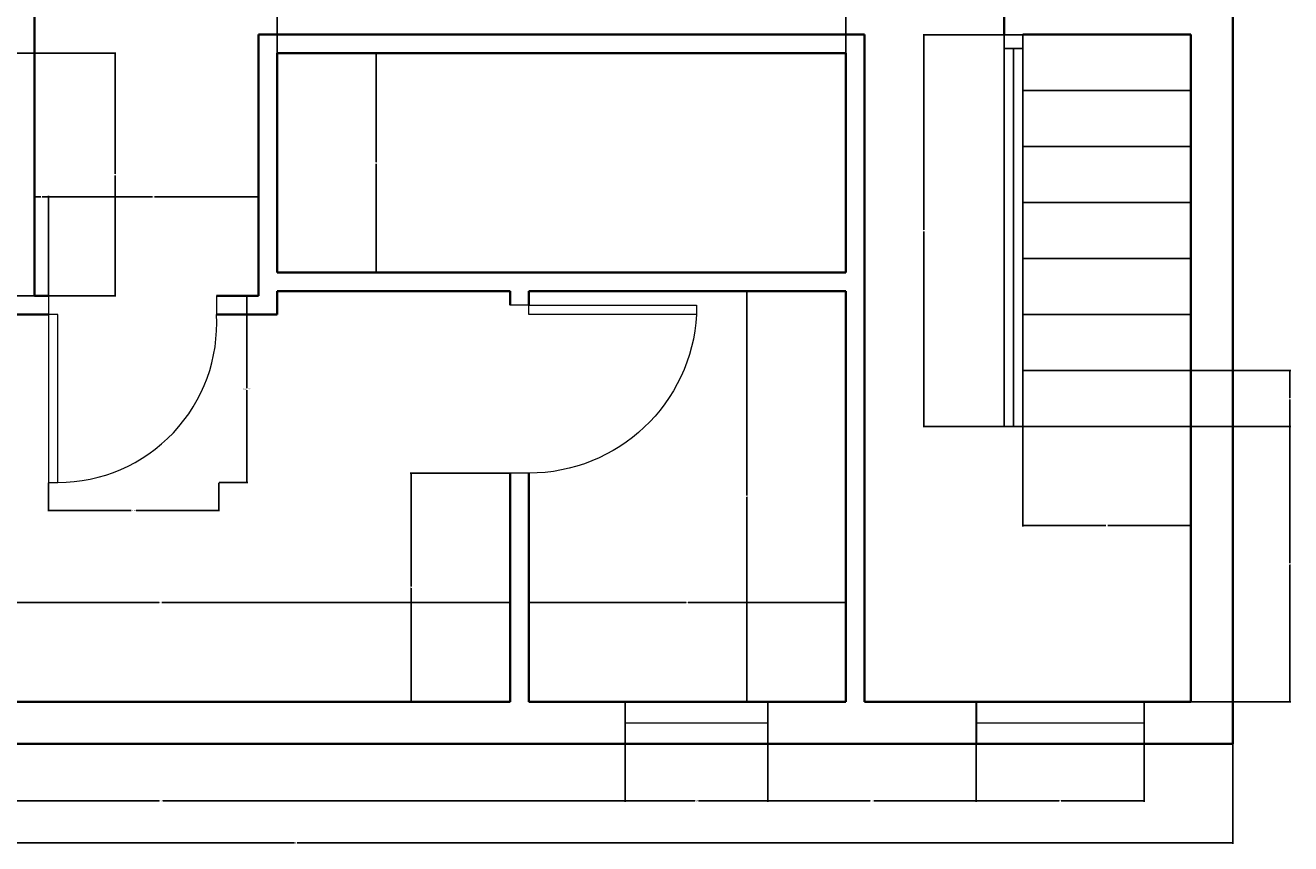
# Model space of a CAD drawing. Units: inches. Extents: x 2345 to 2781, y 2622 to 3032.
# Tile 2 of 3: x 2509 to 2781, y 2622 to 2798. Entities that reach past the tile are written whole.
import ezdxf

# ---------------------------------------------------------------- set-up
doc = ezdxf.new("R2010")
doc.units = ezdxf.units.IN
for name, color, linetype, lineweight in [('A-ANNO-DIMS', 2, 'Continuous', 18), ('A-DOOR', 3, 'Continuous', 18), ('A-FLOR-STRS', 7, 'Continuous', 25), ('A-GLAZ', 4, 'Continuous', 18), ('A-WALL', 7, 'Continuous', 35)]:
    doc.layers.add(name, color=color, linetype=linetype, lineweight=lineweight)
doc.styles.get("Standard").update_dxf_attribs({"font": 'arial.ttf'})
doc.dimstyles.get("Standard").update_dxf_attribs({"dimtxt": 0.18, "dimasz": 0.18, "dimexe": 0.18, "dimexo": 0.0625, "dimgap": 0.09, "dimtad": 0, "dimtih": 1, "dimtoh": 1, "dimdec": 4, "dimzin": 0, "dimdsep": 46, "dimtxsty": 'Standard', "dimcen": 0.09, "dimadec": 0, "dimazin": 0, "dimtfac": 1, "dimtdec": 4, "dimtofl": 0, "dimtmove": 0, "dimatfit": 3, "dimfxl": 1, "dimtolj": 1, "dimtzin": 0, "dimarcsym": 0})

# ---------------------------------------------------------------- blocks, each defined once
blk = doc.blocks.new('DOOR-36IN-SWING-A')
for p, q in [((36, 40), (34, 40)), ((34, 40), (34, 4)), ((36, 4), (36, 40)), ((0, 4), (0, 0)), ((34, 4), (36, 4)), ((36, 4), (36, 0))]:
    blk.add_line(p, q)
blk.add_arc((36.06, 4), 36.06, 93.2732, 180)
blk = doc.blocks.new('DOOR-36IN-SWING-B')
for p, q in [((0, 40), (0, 36)), ((36, 40), (36, 36)), ((0, 36), (0, 0)), ((2, 36), (0, 36)), ((2, 0), (2, 36)), ((0, 0), (2, 0))]:
    blk.add_line(p, q)
blk.add_arc((2, 34.06), 34.06, 270, 3.2732)
blk = doc.blocks.new('*D6')
at = {"layer": 'A-ANNO-DIMS', "color": 0, "lineweight": -2, "transparency": 16777216}
for p, q in [((2550.87, 2739.8), (2556.99, 2739.8)), ((2556.81, 2739.62), (2556.81, 2719.99)), ((2556.81, 2699.98), (2556.81, 2719.62)), ((2550.87, 2699.8), (2556.99, 2699.8))]:
    blk.add_line(p, q, dxfattribs=at)
at = {"layer": 'A-ANNO-DIMS', "color": 0, "transparency": 16777216}
for points in [[(2556.78, 2739.62), (2556.84, 2739.62), (2556.81, 2739.8)], [(2556.78, 2699.98), (2556.84, 2699.98), (2556.81, 2699.8)]]:
    blk.add_solid(points, dxfattribs=at)
at = {"layer": 'Defpoints', "color": 0, "transparency": 16777216}
for p in [(2550.81, 2739.8), (2556.81, 2739.8), (2550.81, 2699.8)]:
    blk.add_point(p, dxfattribs=at)
at = {"layer": 'A-ANNO-DIMS', "color": 0, "transparency": 16777216, "insert": (2556.81, 2719.8), "char_height": 0.18, "attachment_point": 5}
blk.add_mtext('\\A1;DOOR B 40 TYP.', dxfattribs=at)
blk = doc.blocks.new('*D7')
at = {"layer": 'A-ANNO-DIMS', "color": 0, "lineweight": -2, "transparency": 16777216}
for p, q in [((2514.27, 2699.74), (2514.27, 2693.62)), ((2550.81, 2699.74), (2550.81, 2693.62)), ((2514.45, 2693.8), (2532.01, 2693.8)), ((2550.63, 2693.8), (2533.07, 2693.8))]:
    blk.add_line(p, q, dxfattribs=at)
at = {"layer": 'A-ANNO-DIMS', "color": 0, "transparency": 16777216}
for points in [[(2514.45, 2693.83), (2514.45, 2693.77), (2514.27, 2693.8)], [(2550.63, 2693.83), (2550.63, 2693.77), (2550.81, 2693.8)]]:
    blk.add_solid(points, dxfattribs=at)
at = {"layer": 'Defpoints', "color": 0, "transparency": 16777216}
for p in [(2514.27, 2699.8), (2550.81, 2699.8), (2550.81, 2693.8)]:
    blk.add_point(p, dxfattribs=at)
at = {"layer": 'A-ANNO-DIMS', "color": 0, "transparency": 16777216, "insert": (2532.54, 2693.8), "char_height": 0.18, "attachment_point": 5}
blk.add_mtext('\\A1;37 TYP.', dxfattribs=at)
blk = doc.blocks.new('*D10')
at = {"layer": 'A-ANNO-DIMS', "color": 0, "lineweight": -2, "transparency": 16777216}
for p, q in [((2366.27, 2643.74), (2366.27, 2622.37)), ((2768.27, 2643.74), (2768.27, 2622.37)), ((2366.45, 2622.55), (2566.98, 2622.55)), ((2768.09, 2622.55), (2567.56, 2622.55))]:
    blk.add_line(p, q, dxfattribs=at)
at = {"layer": 'A-ANNO-DIMS', "color": 0, "transparency": 16777216}
for points in [[(2366.45, 2622.58), (2366.45, 2622.52), (2366.27, 2622.55)], [(2768.09, 2622.58), (2768.09, 2622.52), (2768.27, 2622.55)]]:
    blk.add_solid(points, dxfattribs=at)
at = {"layer": 'Defpoints', "color": 0, "transparency": 16777216}
for p in [(2366.27, 2643.8), (2768.27, 2643.8), (2768.27, 2622.55)]:
    blk.add_point(p, dxfattribs=at)
at = {"layer": 'A-ANNO-DIMS', "color": 0, "transparency": 16777216, "insert": (2567.27, 2622.55), "char_height": 0.18, "attachment_point": 5}
blk.add_mtext('\\A1;402', dxfattribs=at)
blk = doc.blocks.new('*D34')
at = {"layer": 'A-ANNO-DIMS', "color": 0, "lineweight": -2, "transparency": 16777216}
for p, q in [((2507.33, 2791.8), (2528.7, 2791.8)), ((2528.52, 2791.62), (2528.52, 2765.98)), ((2528.52, 2739.98), (2528.52, 2765.62)), ((2507.33, 2739.8), (2528.7, 2739.8))]:
    blk.add_line(p, q, dxfattribs=at)
at = {"layer": 'A-ANNO-DIMS', "color": 0, "transparency": 16777216}
for points in [[(2528.49, 2791.62), (2528.55, 2791.62), (2528.52, 2791.8)], [(2528.49, 2739.98), (2528.55, 2739.98), (2528.52, 2739.8)]]:
    blk.add_solid(points, dxfattribs=at)
at = {"layer": 'Defpoints', "color": 0, "transparency": 16777216}
for p in [(2507.27, 2791.8), (2507.27, 2739.8), (2528.52, 2739.8)]:
    blk.add_point(p, dxfattribs=at)
at = {"layer": 'A-ANNO-DIMS', "color": 0, "transparency": 16777216, "insert": (2528.52, 2765.8), "char_height": 0.18, "attachment_point": 5}
blk.add_mtext('\\A1;52', dxfattribs=at)
blk = doc.blocks.new('*D36')
at = {"layer": 'A-ANNO-DIMS', "color": 0, "lineweight": -2, "transparency": 16777216}
for p, q in [((2514.27, 2739.87), (2514.27, 2761.23)), ((2514.45, 2761.05), (2536.55, 2761.05)), ((2559.09, 2761.05), (2537, 2761.05)), ((2559.27, 2739.87), (2559.27, 2761.23))]:
    blk.add_line(p, q, dxfattribs=at)
at = {"layer": 'A-ANNO-DIMS', "color": 0, "transparency": 16777216}
for points in [[(2514.45, 2761.08), (2514.45, 2761.02), (2514.27, 2761.05)], [(2559.09, 2761.08), (2559.09, 2761.02), (2559.27, 2761.05)]]:
    blk.add_solid(points, dxfattribs=at)
at = {"layer": 'Defpoints', "color": 0, "transparency": 16777216}
for p in [(2559.27, 2761.05), (2514.27, 2739.8), (2559.27, 2739.8)]:
    blk.add_point(p, dxfattribs=at)
at = {"layer": 'A-ANNO-DIMS', "color": 0, "transparency": 16777216, "insert": (2536.77, 2761.05), "char_height": 0.18, "attachment_point": 5}
blk.add_mtext('\\A1;45', dxfattribs=at)
blk = doc.blocks.new('*D38')
at = {"layer": 'A-ANNO-DIMS', "color": 0, "lineweight": -2, "transparency": 16777216}
for p, q in [((2511.27, 2739.87), (2511.27, 2761.23)), ((2511.45, 2761.05), (2512.62, 2761.05)), ((2514.09, 2761.05), (2512.92, 2761.05)), ((2514.27, 2739.87), (2514.27, 2761.23))]:
    blk.add_line(p, q, dxfattribs=at)
at = {"layer": 'A-ANNO-DIMS', "color": 0, "transparency": 16777216}
for points in [[(2511.45, 2761.08), (2511.45, 2761.02), (2511.27, 2761.05)], [(2514.09, 2761.08), (2514.09, 2761.02), (2514.27, 2761.05)]]:
    blk.add_solid(points, dxfattribs=at)
at = {"layer": 'Defpoints', "color": 0, "transparency": 16777216}
for p in [(2514.27, 2761.05), (2511.27, 2739.8), (2514.27, 2739.8)]:
    blk.add_point(p, dxfattribs=at)
at = {"layer": 'A-ANNO-DIMS', "color": 0, "transparency": 16777216, "insert": (2512.77, 2761.05), "char_height": 0.18, "attachment_point": 5}
blk.add_mtext('\\A1;3', dxfattribs=at)
blk = doc.blocks.new('*D39')
at = {"layer": 'A-ANNO-DIMS', "color": 0, "lineweight": -2, "transparency": 16777216}
for p, q in [((2563.27, 2791.87), (2563.27, 2813.23)), ((2563.45, 2813.05), (2623.99, 2813.05)), ((2685.09, 2813.05), (2624.55, 2813.05)), ((2685.27, 2791.87), (2685.27, 2813.23))]:
    blk.add_line(p, q, dxfattribs=at)
at = {"layer": 'A-ANNO-DIMS', "color": 0, "transparency": 16777216}
for points in [[(2563.45, 2813.08), (2563.45, 2813.02), (2563.27, 2813.05)], [(2685.09, 2813.08), (2685.09, 2813.02), (2685.27, 2813.05)]]:
    blk.add_solid(points, dxfattribs=at)
at = {"layer": 'Defpoints', "color": 0, "transparency": 16777216}
for p in [(2685.27, 2813.05), (2563.27, 2791.8), (2685.27, 2791.8)]:
    blk.add_point(p, dxfattribs=at)
at = {"layer": 'A-ANNO-DIMS', "color": 0, "transparency": 16777216, "insert": (2624.27, 2813.05), "char_height": 0.18, "attachment_point": 5}
blk.add_mtext('\\A1;122', dxfattribs=at)
blk = doc.blocks.new('*D40')
at = {"layer": 'A-ANNO-DIMS', "color": 0, "lineweight": -2, "transparency": 16777216}
for p, q in [((2563.334411, 2791.80295), (2584.701911, 2791.80295)), ((2584.521911, 2791.62295), (2584.521911, 2768.48295)), ((2584.521911, 2744.98295), (2584.521911, 2768.12295)), ((2563.334411, 2744.80295), (2584.701911, 2744.80295))]:
    blk.add_line(p, q, dxfattribs=at)
at = {"layer": 'A-ANNO-DIMS', "color": 0, "transparency": 16777216}
for points in [[(2584.491911, 2791.62295), (2584.551911, 2791.62295), (2584.521911, 2791.80295)], [(2584.491911, 2744.98295), (2584.551911, 2744.98295), (2584.521911, 2744.80295)]]:
    blk.add_solid(points, dxfattribs=at)
at = {"layer": 'Defpoints', "color": 0, "transparency": 16777216}
for p in [(2563.271911, 2791.80295), (2563.271911, 2744.80295), (2584.521911, 2744.80295)]:
    blk.add_point(p, dxfattribs=at)
at = {"layer": 'A-ANNO-DIMS', "color": 0, "transparency": 16777216, "insert": (2584.521911, 2768.30295), "char_height": 0.18, "attachment_point": 5}
blk.add_mtext('\\A1;47', dxfattribs=at)
blk = doc.blocks.new('*D45')
at = {"layer": 'A-ANNO-DIMS', "color": 0, "lineweight": -2, "transparency": 16777216}
for p, q in [((2723.27, 2711.74), (2723.27, 2690.37)), ((2759.27, 2711.74), (2759.27, 2690.37)), ((2723.45, 2690.55), (2741.05, 2690.55)), ((2759.09, 2690.55), (2741.49, 2690.55))]:
    blk.add_line(p, q, dxfattribs=at)
at = {"layer": 'A-ANNO-DIMS', "color": 0, "transparency": 16777216}
for points in [[(2723.45, 2690.58), (2723.45, 2690.52), (2723.27, 2690.55)], [(2759.09, 2690.58), (2759.09, 2690.52), (2759.27, 2690.55)]]:
    blk.add_solid(points, dxfattribs=at)
at = {"layer": 'Defpoints', "color": 0, "transparency": 16777216}
for p in [(2723.27, 2711.8), (2759.27, 2711.8), (2723.27, 2690.55)]:
    blk.add_point(p, dxfattribs=at)
at = {"layer": 'A-ANNO-DIMS', "color": 0, "transparency": 16777216, "insert": (2741.27, 2690.55), "char_height": 0.18, "attachment_point": 5}
blk.add_mtext('\\A1;36', dxfattribs=at)
blk = doc.blocks.new('*D46')
at = {"layer": 'A-ANNO-DIMS', "color": 0, "lineweight": -2, "transparency": 16777216}
for p, q in [((2723.21, 2795.8), (2701.84, 2795.8)), ((2702.02, 2795.62), (2702.02, 2753.98)), ((2702.02, 2711.98), (2702.02, 2753.62)), ((2723.21, 2711.8), (2701.84, 2711.8))]:
    blk.add_line(p, q, dxfattribs=at)
at = {"layer": 'A-ANNO-DIMS', "color": 0, "transparency": 16777216}
for points in [[(2701.99, 2795.62), (2702.05, 2795.62), (2702.02, 2795.8)], [(2701.99, 2711.98), (2702.05, 2711.98), (2702.02, 2711.8)]]:
    blk.add_solid(points, dxfattribs=at)
at = {"layer": 'Defpoints', "color": 0, "transparency": 16777216}
for p in [(2702.02, 2795.8), (2723.27, 2795.8), (2723.27, 2711.8)]:
    blk.add_point(p, dxfattribs=at)
at = {"layer": 'A-ANNO-DIMS', "color": 0, "transparency": 16777216, "insert": (2702.02, 2753.8), "char_height": 0.18, "attachment_point": 5}
blk.add_mtext('\\A1;84', dxfattribs=at)
blk = doc.blocks.new('*D47')
at = {"layer": 'A-ANNO-DIMS', "color": 0, "lineweight": -2, "transparency": 16777216}
for p, q in [((2759.33, 2723.8), (2780.7, 2723.8)), ((2780.52, 2723.62), (2780.52, 2717.98)), ((2780.52, 2711.98), (2780.52, 2717.62)), ((2759.33, 2711.8), (2780.7, 2711.8))]:
    blk.add_line(p, q, dxfattribs=at)
at = {"layer": 'A-ANNO-DIMS', "color": 0, "transparency": 16777216}
for points in [[(2780.49, 2723.62), (2780.55, 2723.62), (2780.52, 2723.8)], [(2780.49, 2711.98), (2780.55, 2711.98), (2780.52, 2711.8)]]:
    blk.add_solid(points, dxfattribs=at)
at = {"layer": 'Defpoints', "color": 0, "transparency": 16777216}
for p in [(2759.27, 2723.8), (2759.27, 2711.8), (2780.52, 2711.8)]:
    blk.add_point(p, dxfattribs=at)
at = {"layer": 'A-ANNO-DIMS', "color": 0, "transparency": 16777216, "insert": (2780.52, 2717.8), "char_height": 0.18, "attachment_point": 5}
blk.add_mtext('\\A1;12', dxfattribs=at)
blk = doc.blocks.new('*D48')
at = {"layer": 'A-ANNO-DIMS', "color": 0, "lineweight": -2, "transparency": 16777216}
for p, q in [((2759.33, 2711.8), (2780.7, 2711.8)), ((2780.52, 2711.62), (2780.52, 2682.48)), ((2780.52, 2652.98), (2780.52, 2682.12)), ((2759.33, 2652.8), (2780.7, 2652.8))]:
    blk.add_line(p, q, dxfattribs=at)
at = {"layer": 'A-ANNO-DIMS', "color": 0, "transparency": 16777216}
for points in [[(2780.49, 2711.62), (2780.55, 2711.62), (2780.52, 2711.8)], [(2780.49, 2652.98), (2780.55, 2652.98), (2780.52, 2652.8)]]:
    blk.add_solid(points, dxfattribs=at)
at = {"layer": 'Defpoints', "color": 0, "transparency": 16777216}
for p in [(2759.27, 2711.8), (2759.27, 2652.8), (2780.52, 2652.8)]:
    blk.add_point(p, dxfattribs=at)
at = {"layer": 'A-ANNO-DIMS', "color": 0, "transparency": 16777216, "insert": (2780.52, 2682.3), "char_height": 0.18, "attachment_point": 5}
blk.add_mtext('\\A1;59', dxfattribs=at)
blk = doc.blocks.new('*D52')
at = {"layer": 'A-ANNO-DIMS', "color": 0, "lineweight": -2, "transparency": 16777216}
for p, q in [((2463.27, 2652.87), (2463.27, 2674.23)), ((2463.45, 2674.05), (2537.99, 2674.05)), ((2613.09, 2674.05), (2538.55, 2674.05)), ((2613.27, 2652.87), (2613.27, 2674.23))]:
    blk.add_line(p, q, dxfattribs=at)
at = {"layer": 'A-ANNO-DIMS', "color": 0, "transparency": 16777216}
for points in [[(2463.45, 2674.08), (2463.45, 2674.02), (2463.27, 2674.05)], [(2613.09, 2674.08), (2613.09, 2674.02), (2613.27, 2674.05)]]:
    blk.add_solid(points, dxfattribs=at)
at = {"layer": 'Defpoints', "color": 0, "transparency": 16777216}
for p in [(2613.27, 2674.05), (2463.27, 2652.8), (2613.27, 2652.8)]:
    blk.add_point(p, dxfattribs=at)
at = {"layer": 'A-ANNO-DIMS', "color": 0, "transparency": 16777216, "insert": (2538.27, 2674.05), "char_height": 0.18, "attachment_point": 5}
blk.add_mtext('\\A1;150', dxfattribs=at)
blk = doc.blocks.new('*D53')
at = {"layer": 'A-ANNO-DIMS', "color": 0, "lineweight": -2, "transparency": 16777216}
for p, q in [((2617.27, 2652.87), (2617.27, 2674.23)), ((2617.45, 2674.05), (2651.05, 2674.05)), ((2685.09, 2674.05), (2651.49, 2674.05)), ((2685.27, 2652.87), (2685.27, 2674.23))]:
    blk.add_line(p, q, dxfattribs=at)
at = {"layer": 'A-ANNO-DIMS', "color": 0, "transparency": 16777216}
for points in [[(2617.45, 2674.08), (2617.45, 2674.02), (2617.27, 2674.05)], [(2685.09, 2674.08), (2685.09, 2674.02), (2685.27, 2674.05)]]:
    blk.add_solid(points, dxfattribs=at)
at = {"layer": 'Defpoints', "color": 0, "transparency": 16777216}
for p in [(2685.27, 2674.05), (2617.27, 2652.8), (2685.27, 2652.8)]:
    blk.add_point(p, dxfattribs=at)
at = {"layer": 'A-ANNO-DIMS', "color": 0, "transparency": 16777216, "insert": (2651.27, 2674.05), "char_height": 0.18, "attachment_point": 5}
blk.add_mtext('\\A1;68', dxfattribs=at)
blk = doc.blocks.new('*D54')
at = {"layer": 'A-ANNO-DIMS', "color": 0, "lineweight": -2, "transparency": 16777216}
for p, q in [((2685.21, 2740.8), (2663.84, 2740.8)), ((2664.02, 2740.62), (2664.02, 2696.98)), ((2664.02, 2652.98), (2664.02, 2696.62)), ((2685.21, 2652.8), (2663.84, 2652.8))]:
    blk.add_line(p, q, dxfattribs=at)
at = {"layer": 'A-ANNO-DIMS', "color": 0, "transparency": 16777216}
for points in [[(2663.99, 2740.62), (2664.05, 2740.62), (2664.02, 2740.8)], [(2663.99, 2652.98), (2664.05, 2652.98), (2664.02, 2652.8)]]:
    blk.add_solid(points, dxfattribs=at)
at = {"layer": 'Defpoints', "color": 0, "transparency": 16777216}
for p in [(2664.02, 2740.8), (2685.27, 2740.8), (2685.27, 2652.8)]:
    blk.add_point(p, dxfattribs=at)
at = {"layer": 'A-ANNO-DIMS', "color": 0, "transparency": 16777216, "insert": (2664.02, 2696.8), "char_height": 0.18, "attachment_point": 5}
blk.add_mtext('\\A1;88', dxfattribs=at)
blk = doc.blocks.new('*D56')
at = {"layer": 'A-ANNO-DIMS', "color": 0, "lineweight": -2, "transparency": 16777216}
for p, q in [((2613.21, 2701.8), (2591.84, 2701.8)), ((2592.02, 2701.62), (2592.02, 2677.48)), ((2592.02, 2652.98), (2592.02, 2677.12)), ((2613.21, 2652.8), (2591.84, 2652.8))]:
    blk.add_line(p, q, dxfattribs=at)
at = {"layer": 'A-ANNO-DIMS', "color": 0, "transparency": 16777216}
for points in [[(2591.99, 2701.62), (2592.05, 2701.62), (2592.02, 2701.8)], [(2591.99, 2652.98), (2592.05, 2652.98), (2592.02, 2652.8)]]:
    blk.add_solid(points, dxfattribs=at)
at = {"layer": 'Defpoints', "color": 0, "transparency": 16777216}
for p in [(2592.02, 2701.8), (2613.27, 2701.8), (2613.27, 2652.8)]:
    blk.add_point(p, dxfattribs=at)
at = {"layer": 'A-ANNO-DIMS', "color": 0, "transparency": 16777216, "insert": (2592.02, 2677.3), "char_height": 0.18, "attachment_point": 5}
blk.add_mtext('\\A1;49', dxfattribs=at)
blk = doc.blocks.new('*D59')
at = {"layer": 'A-ANNO-DIMS', "color": 0, "lineweight": -2, "transparency": 16777216}
for p, q in [((2438.77, 2652.74), (2438.77, 2631.37)), ((2637.97, 2652.74), (2637.97, 2631.37)), ((2438.95, 2631.55), (2537.98, 2631.55)), ((2637.79, 2631.55), (2538.75, 2631.55))]:
    blk.add_line(p, q, dxfattribs=at)
at = {"layer": 'A-ANNO-DIMS', "color": 0, "transparency": 16777216}
for points in [[(2438.95, 2631.58), (2438.95, 2631.52), (2438.77, 2631.55)], [(2637.79, 2631.58), (2637.79, 2631.52), (2637.97, 2631.55)]]:
    blk.add_solid(points, dxfattribs=at)
at = {"layer": 'Defpoints', "color": 0, "transparency": 16777216}
for p in [(2438.77, 2652.8), (2637.97, 2652.8), (2438.77, 2631.55)]:
    blk.add_point(p, dxfattribs=at)
at = {"layer": 'A-ANNO-DIMS', "color": 0, "transparency": 16777216, "insert": (2538.37, 2631.55), "char_height": 0.18, "attachment_point": 5}
blk.add_mtext('\\A1;199.2', dxfattribs=at)
blk = doc.blocks.new('*D60')
at = {"layer": 'A-ANNO-DIMS', "color": 0, "lineweight": -2, "transparency": 16777216}
for p, q in [((2637.97, 2652.74), (2637.97, 2631.37)), ((2668.54, 2652.74), (2668.54, 2631.37)), ((2638.15, 2631.55), (2652.86, 2631.55)), ((2668.36, 2631.55), (2653.65, 2631.55))]:
    blk.add_line(p, q, dxfattribs=at)
at = {"layer": 'A-ANNO-DIMS', "color": 0, "transparency": 16777216}
for points in [[(2638.15, 2631.58), (2638.15, 2631.52), (2637.97, 2631.55)], [(2668.36, 2631.58), (2668.36, 2631.52), (2668.54, 2631.55)]]:
    blk.add_solid(points, dxfattribs=at)
at = {"layer": 'Defpoints', "color": 0, "transparency": 16777216}
for p in [(2637.97, 2652.8), (2668.54, 2652.8), (2637.97, 2631.55)]:
    blk.add_point(p, dxfattribs=at)
at = {"layer": 'A-ANNO-DIMS', "color": 0, "transparency": 16777216, "insert": (2653.25, 2631.55), "char_height": 0.18, "attachment_point": 5}
blk.add_mtext('\\A1;30.57', dxfattribs=at)
blk = doc.blocks.new('*D61')
at = {"layer": 'A-ANNO-DIMS', "color": 0, "lineweight": -2, "transparency": 16777216}
for p, q in [((2668.54, 2652.74), (2668.54, 2631.37)), ((2713.27, 2652.74), (2713.27, 2631.37)), ((2668.72, 2631.55), (2690.51, 2631.55)), ((2713.09, 2631.55), (2691.3, 2631.55))]:
    blk.add_line(p, q, dxfattribs=at)
at = {"layer": 'A-ANNO-DIMS', "color": 0, "transparency": 16777216}
for points in [[(2668.72, 2631.58), (2668.72, 2631.52), (2668.54, 2631.55)], [(2713.09, 2631.58), (2713.09, 2631.52), (2713.27, 2631.55)]]:
    blk.add_solid(points, dxfattribs=at)
at = {"layer": 'Defpoints', "color": 0, "transparency": 16777216}
for p in [(2668.54, 2652.8), (2713.27, 2652.8), (2668.54, 2631.55)]:
    blk.add_point(p, dxfattribs=at)
at = {"layer": 'A-ANNO-DIMS', "color": 0, "transparency": 16777216, "insert": (2690.9, 2631.55), "char_height": 0.18, "attachment_point": 5}
blk.add_mtext('\\A1;44.74', dxfattribs=at)
blk = doc.blocks.new('*D62')
at = {"layer": 'A-ANNO-DIMS', "color": 0, "lineweight": -2, "transparency": 16777216}
for p, q in [((2713.27, 2652.74), (2713.27, 2631.37)), ((2749.27, 2652.74), (2749.27, 2631.37)), ((2713.45, 2631.55), (2731.05, 2631.55)), ((2749.09, 2631.55), (2731.49, 2631.55))]:
    blk.add_line(p, q, dxfattribs=at)
at = {"layer": 'A-ANNO-DIMS', "color": 0, "transparency": 16777216}
for points in [[(2713.45, 2631.58), (2713.45, 2631.52), (2713.27, 2631.55)], [(2749.09, 2631.58), (2749.09, 2631.52), (2749.27, 2631.55)]]:
    blk.add_solid(points, dxfattribs=at)
at = {"layer": 'Defpoints', "color": 0, "transparency": 16777216}
for p in [(2713.27, 2652.8), (2749.27, 2652.8), (2713.27, 2631.55)]:
    blk.add_point(p, dxfattribs=at)
at = {"layer": 'A-ANNO-DIMS', "color": 0, "transparency": 16777216, "insert": (2731.27, 2631.55), "char_height": 0.18, "attachment_point": 5}
blk.add_mtext('\\A1;36', dxfattribs=at)

msp = doc.modelspace()

# ---------------------------------------------------------------- linework, layer by layer
at = {"layer": 'A-FLOR-STRS'}
for p, q in [((2719.2719, 2711.8029), (2719.2719, 2795.8029)), ((2723.2719, 2711.8029), (2723.2719, 2795.8029)), ((2723.2719, 2792.803), (2719.2719, 2792.803)), ((2721.2719, 2792.803), (2721.2719, 2711.8029)), ((2759.2719, 2783.803), (2723.2719, 2783.803)), ((2759.2719, 2771.803), (2723.2719, 2771.803)), ((2759.2719, 2759.803), (2723.2719, 2759.803)), ((2759.2719, 2747.803), (2723.2719, 2747.803)), ((2759.2719, 2735.803), (2723.2719, 2735.803)), ((2759.2719, 2723.8029), (2723.2719, 2723.8029)), ((2723.2719, 2711.8029), (2719.2719, 2711.8029)), ((2759.2719, 2711.8029), (2723.2719, 2711.8029))]:
    msp.add_line(p, q, dxfattribs=at)
at = {"layer": 'A-GLAZ'}
for p, q in [((2637.9676, 2652.8029), (2637.9676, 2643.8029)), ((2668.5362, 2652.8029), (2668.5362, 2643.8029)), ((2713.2719, 2652.8029), (2713.2719, 2643.8029)), ((2749.2719, 2652.8029), (2749.2719, 2643.8029)), ((2637.9676, 2648.303), (2668.5362, 2648.303)), ((2713.2719, 2648.303), (2749.2719, 2648.303))]:
    msp.add_line(p, q, dxfattribs=at)
at = {"layer": 'A-WALL'}
for p, q in [((2768.2719, 2643.8029), (2768.2719, 3010.803)), ((2511.2719, 2801.803), (2511.2719, 2739.8029)), ((2719.2719, 2799.803), (2719.2719, 2795.8029)), ((2559.2719, 2790.803), (2559.2719, 2795.8029)), ((2559.2719, 2795.8029), (2563.2719, 2795.8029)), ((2689.2719, 2795.8029), (2563.2719, 2795.8029)), ((2689.2719, 2795.8029), (2685.2719, 2795.8029)), ((2689.2719, 2786.803), (2689.2719, 2795.8029)), ((2759.2719, 2795.8029), (2723.2719, 2795.8029)), ((2729.2719, 2795.8029), (2725.2719, 2795.8029)), ((2759.2719, 2652.8029), (2759.2719, 2795.8029)), ((2559.2719, 2790.803), (2559.2719, 2739.8029)), ((2563.2719, 2791.8029), (2685.2719, 2791.8029)), ((2563.2719, 2791.8029), (2563.2719, 2786.803)), ((2685.2719, 2791.8029), (2685.2719, 2790.803)), ((2685.2719, 2790.803), (2685.2719, 2784.8003)), ((2689.2719, 2739.8029), (2689.2719, 2790.803)), ((2563.2719, 2786.803), (2563.2719, 2765.803)), ((2685.2719, 2765.803), (2685.2719, 2786.803)), ((2563.2719, 2761.803), (2563.2719, 2765.803)), ((2685.2719, 2761.803), (2685.2719, 2765.803)), ((2563.2719, 2761.803), (2563.2719, 2744.8029)), ((2685.2719, 2744.8029), (2685.2719, 2761.803)), ((2563.2719, 2744.8029), (2685.2719, 2744.8029)), ((2511.2719, 2739.8029), (2512.8904, 2739.8029)), ((2514.2719, 2739.8029), (2511.2719, 2739.8029)), ((2559.2719, 2739.8029), (2550.2719, 2739.8029)), ((2563.2719, 2740.8029), (2613.2719, 2740.8029)), ((2563.2719, 2740.8029), (2563.2719, 2739.8029)), ((2563.2719, 2739.8029), (2563.2719, 2735.803)), ((2613.2719, 2737.803), (2613.2719, 2740.8029)), ((2617.2719, 2740.8029), (2617.2719, 2737.803)), ((2617.2719, 2740.8029), (2685.2719, 2740.8029)), ((2685.2719, 2739.8029), (2685.2719, 2740.8029)), ((2685.2719, 2739.8029), (2685.2719, 2735.803)), ((2689.2719, 2739.8029), (2689.2719, 2735.803)), ((2759.2719, 2739.8029), (2759.2719, 2732.8897)), ((2507.2719, 2735.803), (2511.7641, 2735.803)), ((2514.2719, 2735.803), (2511.2719, 2735.803)), ((2559.2719, 2735.803), (2550.2719, 2735.803)), ((2563.2719, 2735.803), (2559.2719, 2735.803)), ((2685.2719, 2735.803), (2685.2719, 2652.8029)), ((2689.2719, 2652.8029), (2689.2719, 2735.803)), ((2613.2719, 2701.8029), (2613.2719, 2652.8029)), ((2617.2719, 2701.8029), (2617.2719, 2652.8029)), ((2507.2719, 2652.8029), (2513.846, 2652.8029)), ((2511.2719, 2652.8029), (2613.2719, 2652.8029)), ((2617.2719, 2652.8029), (2631.2719, 2652.8029)), ((2631.2719, 2652.8029), (2638.8468, 2652.8029)), ((2635.2719, 2652.8029), (2685.2719, 2652.8029)), ((2689.2719, 2652.8029), (2759.2719, 2652.8029)), ((2366.2719, 2643.8029), (2768.2719, 2643.8029))]:
    msp.add_line(p, q, dxfattribs=at)

# ---------------------------------------------------------------- block references
at = {"layer": 'A-DOOR'}
msp.add_blockref('DOOR-36IN-SWING-B', (2514.272, 2699.803), dxfattribs=at)
at = {"layer": 'A-DOOR', "extrusion": (0, 0, -1), "zscale": -1, "rotation": 89.99999999999856}
msp.add_blockref('DOOR-36IN-SWING-A', (-2613.272, 2701.803), dxfattribs=at)

# ---------------------------------------------------------------- dimensions: what is measured, and where the dimension line sits
at = {"layer": 'A-ANNO-DIMS'}
for base, p1, p2, picture, middle in [((2685.2719, 2813.0529), (2563.2719, 2791.8029), (2685.2719, 2791.8029), '*D39', (2624.2719, 2813.0529)), ((2514.2719, 2761.0529), (2511.2719, 2739.8029), (2514.2719, 2739.8029), '*D38', (2512.7719, 2761.0529)), ((2685.2719, 2674.0529), (2617.2719, 2652.8029), (2685.2719, 2652.8029), '*D53', (2651.2719, 2674.0529)), ((2768.2719, 2622.5529), (2366.2719, 2643.8029), (2768.2719, 2643.8029), '*D10', (2567.2719, 2622.5529))]:
    dim = msp.add_linear_dim(base=base, p1=p1, p2=p2, dimstyle='Standard', override={"dimdec": 0, "dimlfac": 1, "dimrnd": 0, "dimzin": 0, "dimdsep": 46, "dimlunit": 2}, dxfattribs=at)
    dim.commit()
    dim.dimension.update_dxf_attribs({"geometry": picture, "text_midpoint": middle})
for base, p1, p2, angle, override, picture, middle in [((2702.0219, 2795.8029), (2723.2719, 2711.8029), (2723.2719, 2795.8029), 90, {"dimdec": 0, "dimlfac": 1, "dimrnd": 0, "dimzin": 0, "dimdsep": 46, "dimlunit": 2}, '*D46', (2702.0219, 2753.8029)), ((2528.5219, 2739.8029), (2507.2719, 2791.8029), (2507.2719, 2739.8029), 270, {"dimdec": 0, "dimlfac": 1, "dimrnd": 0, "dimzin": 0, "dimdsep": 46, "dimlunit": 2}, '*D34', (2528.5219, 2765.8029)), ((2584.5219, 2744.8029), (2563.2719, 2791.8029), (2563.2719, 2744.8029), 270, {"dimdec": 0, "dimlfac": 1, "dimrnd": 0, "dimzin": 0, "dimdsep": 46, "dimlunit": 2}, '*D40', (2584.5219, 2768.3029)), ((2559.2719, 2761.0529), (2514.2719, 2739.8029), (2559.2719, 2739.8029), 0, {"dimdec": 0, "dimlfac": 1, "dimrnd": 0, "dimzin": 0, "dimdsep": 46, "dimlunit": 2}, '*D36', (2536.7719, 2761.0529)), ((2664.0219, 2740.8029), (2685.2719, 2652.8029), (2685.2719, 2740.8029), 90, {"dimdec": 0, "dimlfac": 1, "dimrnd": 0, "dimzin": 0, "dimdsep": 46, "dimlunit": 2}, '*D54', (2664.0219, 2696.8029)), ((2780.5219, 2711.8029), (2759.2719, 2723.8029), (2759.2719, 2711.8029), 270, {"dimdec": 0, "dimlfac": 1, "dimrnd": 0, "dimzin": 0, "dimdsep": 46, "dimlunit": 2}, '*D47', (2780.5219, 2717.8029)), ((2723.2719, 2690.5529), (2759.2719, 2711.8029), (2723.2719, 2711.8029), 180, {"dimdec": 0, "dimlfac": 1, "dimrnd": 0, "dimzin": 0, "dimdsep": 46, "dimlunit": 2}, '*D45', (2741.2719, 2690.5529)), ((2780.5219, 2652.8029), (2759.2719, 2711.8029), (2759.2719, 2652.8029), 270, {"dimdec": 0, "dimlfac": 1, "dimrnd": 0, "dimzin": 0, "dimdsep": 46, "dimlunit": 2}, '*D48', (2780.5219, 2682.3029)), ((2592.0219, 2701.8029), (2613.2719, 2652.8029), (2613.2719, 2701.8029), 90, {"dimdec": 0, "dimlfac": 1, "dimrnd": 0, "dimzin": 0, "dimdsep": 46, "dimlunit": 2}, '*D56', (2592.0219, 2677.3029)), ((2613.2719, 2674.0529), (2463.2719, 2652.8029), (2613.2719, 2652.8029), 0, {"dimdec": 0, "dimlfac": 1, "dimrnd": 0, "dimzin": 0, "dimdsep": 46, "dimlunit": 2}, '*D52', (2538.2719, 2674.0529)), ((2438.7687, 2631.5529), (2637.9676, 2652.8029), (2438.7687, 2652.8029), 180, {"dimdec": 1, "dimlfac": 1, "dimrnd": 0, "dimzin": 0, "dimdsep": 46, "dimlunit": 2}, '*D59', (2538.3681, 2631.5529)), ((2637.9676, 2631.5529), (2668.5362, 2652.8029), (2637.9676, 2652.8029), 180, {"dimdec": 2, "dimlfac": 1, "dimrnd": 0, "dimzin": 0, "dimdsep": 46, "dimlunit": 2}, '*D60', (2653.2519, 2631.5529)), ((2668.5362, 2631.5529), (2713.2719, 2652.8029), (2668.5362, 2652.8029), 180, {"dimdec": 2, "dimlfac": 1, "dimrnd": 0, "dimzin": 0, "dimdsep": 46, "dimlunit": 2}, '*D61', (2690.9041, 2631.5529)), ((2713.2719, 2631.5529), (2749.2719, 2652.8029), (2713.2719, 2652.8029), 180, {"dimdec": 0, "dimlfac": 1, "dimrnd": 0, "dimzin": 0, "dimdsep": 46, "dimlunit": 2}, '*D62', (2731.2719, 2631.5529))]:
    dim = msp.add_linear_dim(base=base, p1=p1, p2=p2, angle=angle, dimstyle='Standard', override=override, dxfattribs=at)
    dim.commit()
    dim.dimension.update_dxf_attribs({"geometry": picture, "text_midpoint": middle})
dim = msp.add_linear_dim(base=(2556.8069, 2739.8029), p1=(2550.8069, 2699.803), p2=(2550.8069, 2739.8029), angle=90, text='DOOR B <> TYP.', dimstyle='Standard', override={"dimdec": 0, "dimlfac": 1, "dimrnd": 0, "dimzin": 0, "dimdsep": 46, "dimlunit": 2}, dxfattribs=at)
dim.commit()
dim.dimension.update_dxf_attribs({"geometry": '*D6', "text_midpoint": (2556.8069, 2719.803)})
dim = msp.add_linear_dim(base=(2550.8069, 2693.803), p1=(2514.2719, 2699.803), p2=(2550.8069, 2699.803), text='<> TYP.', dimstyle='Standard', override={"dimdec": 0, "dimlfac": 1, "dimrnd": 0, "dimzin": 0, "dimdsep": 46, "dimlunit": 2}, dxfattribs=at)
dim.commit()
dim.dimension.update_dxf_attribs({"geometry": '*D7', "text_midpoint": (2532.5394, 2693.803)})

doc.saveas('drawing.dxf')
